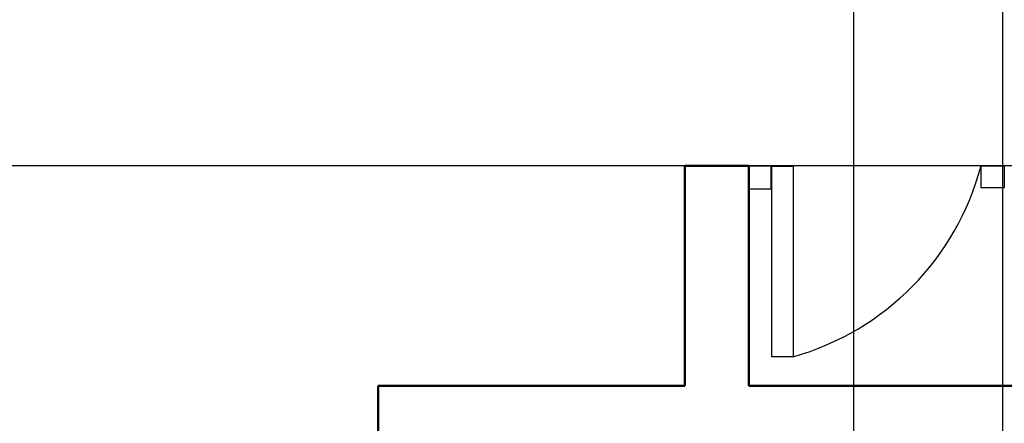
# Model space of a CAD drawing. Units: inches. Extents: x 870 to 1431, y 383 to 1070.
# Tile 3 of 9: x 1091 to 1230, y 604 to 661. Entities that reach past the tile are written whole.
import ezdxf

# ---------------------------------------------------------------- set-up
doc = ezdxf.new("R2010")
doc.units = ezdxf.units.IN
doc.header["$MEASUREMENT"] = 0
for name, color, linetype, lineweight in [('A-ANNO-DIMS', 2, 'Continuous', 18), ('A-DOOR', 3, 'Continuous', 25), ('A-WALL', 7, 'Continuous', 50)]:
    doc.layers.add(name, color=color, linetype=linetype, lineweight=lineweight)
doc.styles.get("Standard").update_dxf_attribs({"font": 'arial.ttf'})
doc.dimstyles.get("Standard").update_dxf_attribs({"dimtxt": 4, "dimasz": 0.18, "dimexe": 0.18, "dimexo": 0.0625, "dimgap": 0.09, "dimtad": 0, "dimtih": 1, "dimtoh": 1, "dimdec": 0, "dimrnd": 6, "dimzin": 0, "dimdsep": 46, "dimlunit": 3, "dimtxsty": 'Standard', "dimcen": 0.09, "dimadec": 0, "dimazin": 0, "dimtfac": 1, "dimtdec": 0, "dimtofl": 0, "dimtmove": 0, "dimatfit": 3, "dimfxl": 1, "dimtolj": 1, "dimtzin": 0, "dimarcsym": 0})

# ---------------------------------------------------------------- blocks, each defined once
blk = doc.blocks.new('*D126')
at = {"layer": 'A-ANNO-DIMS', "color": 0, "lineweight": -2, "transparency": 16777216}
for p, q in [((1168.73, 1009.48), (876.24, 1009.48)), ((876.42, 1009.3), (876.42, 715.17)), ((876.42, 416.77), (876.42, 710.9)), ((1094.63, 416.59), (876.24, 416.59))]:
    blk.add_line(p, q, dxfattribs=at)
at = {"layer": 'A-ANNO-DIMS', "color": 0, "transparency": 16777216}
for points in [[(876.39, 1009.3), (876.45, 1009.3), (876.42, 1009.48)], [(876.39, 416.77), (876.45, 416.77), (876.42, 416.59)]]:
    blk.add_solid(points, dxfattribs=at)
at = {"layer": 'Defpoints', "color": 0, "transparency": 16777216}
for p in [(876.42, 1009.48), (1168.79, 1009.48), (1094.7, 416.59)]:
    blk.add_point(p, dxfattribs=at)
at = {"layer": 'A-ANNO-DIMS', "color": 0, "transparency": 16777216, "insert": (876.42, 713.03), "char_height": 4, "attachment_point": 5}
blk.add_mtext('\\A1;592.9', dxfattribs=at)
blk = doc.blocks.new('*D136')
at = {"layer": 'A-ANNO-DIMS', "color": 0, "lineweight": -2, "transparency": 16777216}
for p, q in [((1208.53, 986.13), (1208.53, 385.26)), ((1229.53, 986.13), (1229.53, 385.26)), ((1208.71, 385.44), (1216.43, 385.44)), ((1229.35, 385.44), (1221.64, 385.44))]:
    blk.add_line(p, q, dxfattribs=at)
at = {"layer": 'A-ANNO-DIMS', "color": 0, "transparency": 16777216}
for points in [[(1208.71, 385.47), (1208.71, 385.41), (1208.53, 385.44)], [(1229.35, 385.47), (1229.35, 385.41), (1229.53, 385.44)]]:
    blk.add_solid(points, dxfattribs=at)
at = {"layer": 'Defpoints', "color": 0, "transparency": 16777216}
for p in [(1208.53, 986.19), (1229.53, 986.19), (1229.53, 385.44)]:
    blk.add_point(p, dxfattribs=at)
at = {"layer": 'A-ANNO-DIMS', "color": 0, "transparency": 16777216, "insert": (1219.03, 385.44), "char_height": 4, "attachment_point": 5}
blk.add_mtext('\\A1;21', dxfattribs=at)
blk = doc.blocks.new('*D140')
at = {"layer": 'A-ANNO-DIMS', "color": 0, "lineweight": -2, "transparency": 16777216}
for p, q in [((1253.73, 676.48), (876.24, 676.48)), ((876.42, 676.3), (876.42, 660.61)), ((876.42, 640.66), (876.42, 656.34)), ((1253.73, 640.48), (876.24, 640.48))]:
    blk.add_line(p, q, dxfattribs=at)
at = {"layer": 'A-ANNO-DIMS', "color": 0, "transparency": 16777216}
for points in [[(876.39, 676.3), (876.45, 676.3), (876.42, 676.48)], [(876.39, 640.66), (876.45, 640.66), (876.42, 640.48)]]:
    blk.add_solid(points, dxfattribs=at)
at = {"layer": 'Defpoints', "color": 0, "transparency": 16777216}
for p in [(876.42, 676.48), (1253.79, 676.48), (1253.79, 640.48)]:
    blk.add_point(p, dxfattribs=at)
at = {"layer": 'A-ANNO-DIMS', "color": 0, "transparency": 16777216, "insert": (876.42, 658.48), "char_height": 4, "attachment_point": 5}
blk.add_mtext('\\A1;36', dxfattribs=at)

msp = doc.modelspace()

# ---------------------------------------------------------------- linework, layer by layer
at = {"layer": 'A-DOOR'}
msp.add_line((1200.0252, 613.5892), (1197.0252, 613.5892), dxfattribs=at)
for points in [[(1193.7907, 637.2078), (1193.7907, 640.4772), (1196.8921, 640.4772), (1196.8921, 637.2078)], [(1229.7793, 637.3734), (1226.51, 637.3734), (1226.51, 640.4748), (1229.7793, 640.4748)]]:
    msp.add_lwpolyline(points, close=True, dxfattribs=at)
msp.add_lwpolyline([(1197.0252, 613.5892), (1197.0252, 640.4249), (1200.0252, 640.4249), (1200.0252, 613.5892)], dxfattribs=at)
msp.add_arc((1189.7597, 650.1894), 38.0126, 285.667489, 345.192997, dxfattribs=at)
at = {"layer": 'A-WALL'}
for p, q in [((1184.7907, 640.4772), (1193.7907, 640.4772)), ((1184.7907, 640.4772), (1184.7907, 609.4772)), ((1193.7907, 640.4772), (1193.7907, 609.4772)), ((1141.5753, 609.4772), (1141.5753, 600.4772)), ((1141.5753, 609.4772), (1184.7907, 609.4772)), ((1193.7907, 609.4772), (1238.7907, 609.4772))]:
    msp.add_line(p, q, dxfattribs=at)

# ---------------------------------------------------------------- dimensions: what is measured, and where the dimension line sits
at = {"layer": 'A-ANNO-DIMS'}
for base, p1, p2, override, picture, middle in [((876.4215, 1009.4772), (1094.6967, 416.59), (1168.7907, 1009.4772), {"dimdec": 1, "dimlfac": 1, "dimrnd": 0, "dimzin": 0, "dimdsep": 46, "dimlunit": 2}, '*D126', (876.4215, 713.0336)), ((876.4215, 676.4772), (1253.7907, 640.4772), (1253.7907, 676.4772), {"dimdec": 0, "dimlfac": 1, "dimrnd": 0, "dimzin": 0, "dimdsep": 46, "dimlunit": 2}, '*D140', (876.4215, 658.4772))]:
    dim = msp.add_linear_dim(base=base, p1=p1, p2=p2, angle=90, dimstyle='Standard', override=override, dxfattribs=at)
    dim.commit()
    dim.dimension.update_dxf_attribs({"geometry": picture, "text_midpoint": middle})
dim = msp.add_linear_dim(base=(1229.5328, 385.44), p1=(1208.5328, 986.1907), p2=(1229.5328, 986.1907), dimstyle='Standard', override={"dimdec": 0, "dimlfac": 1, "dimrnd": 0, "dimzin": 0, "dimdsep": 46, "dimlunit": 2}, dxfattribs=at)
dim.commit()
dim.dimension.update_dxf_attribs({"geometry": '*D136', "text_midpoint": (1219.0328, 385.44)})

doc.saveas('drawing.dxf')
